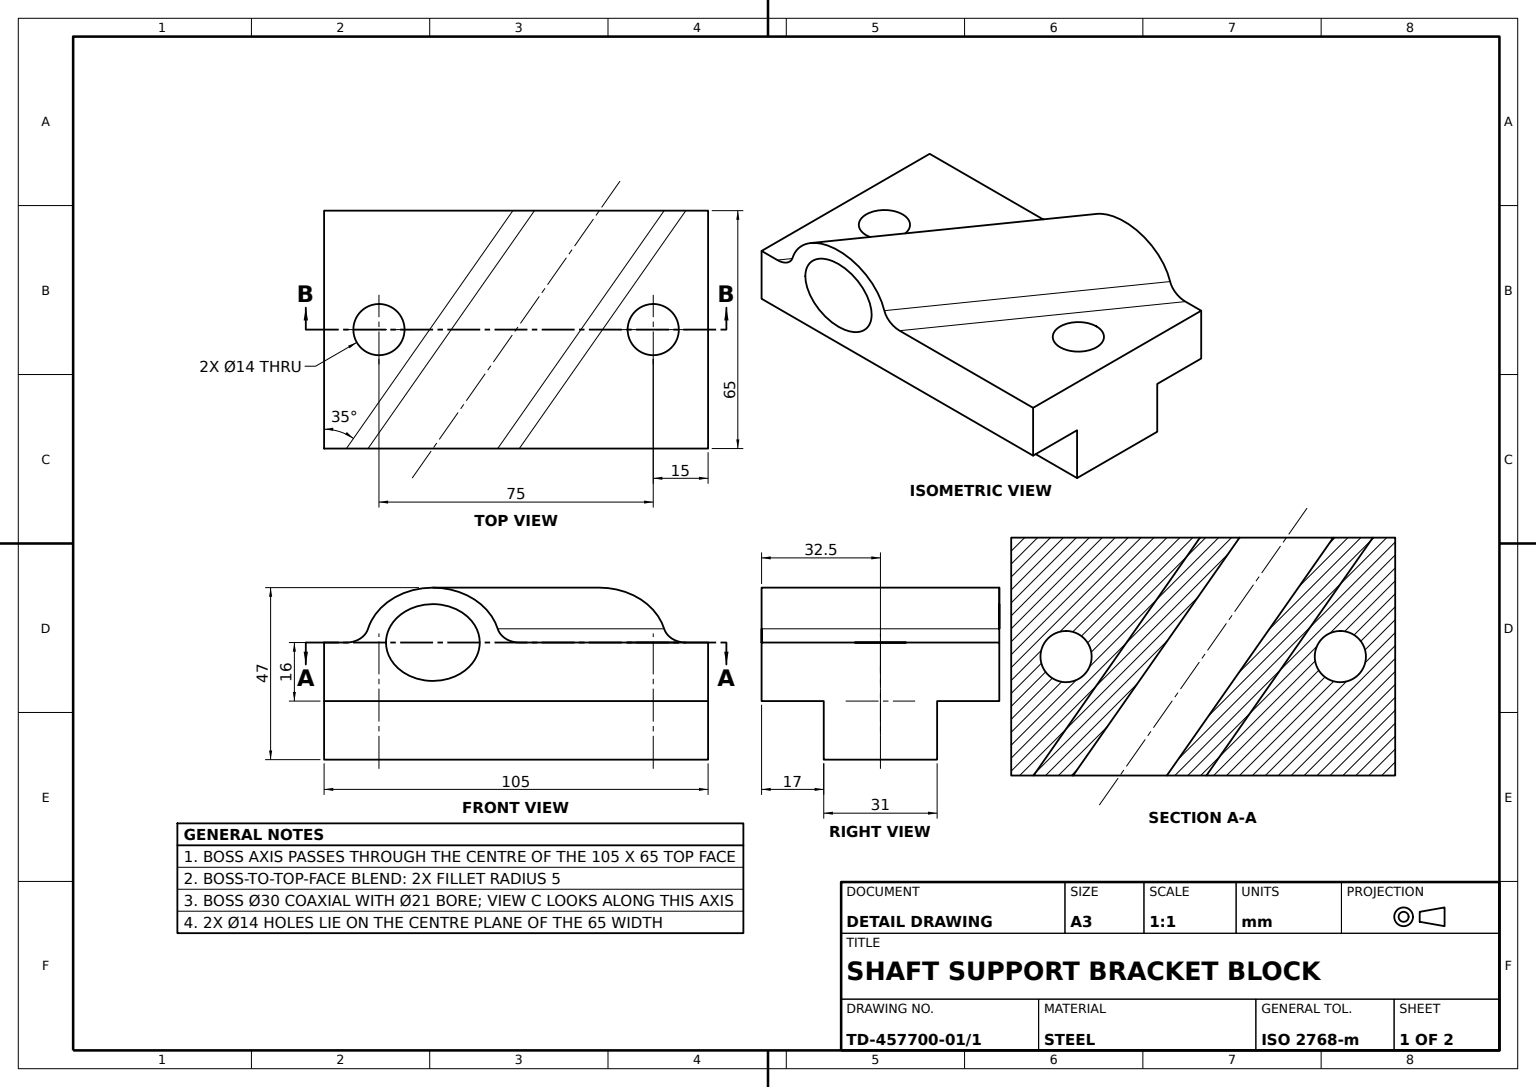
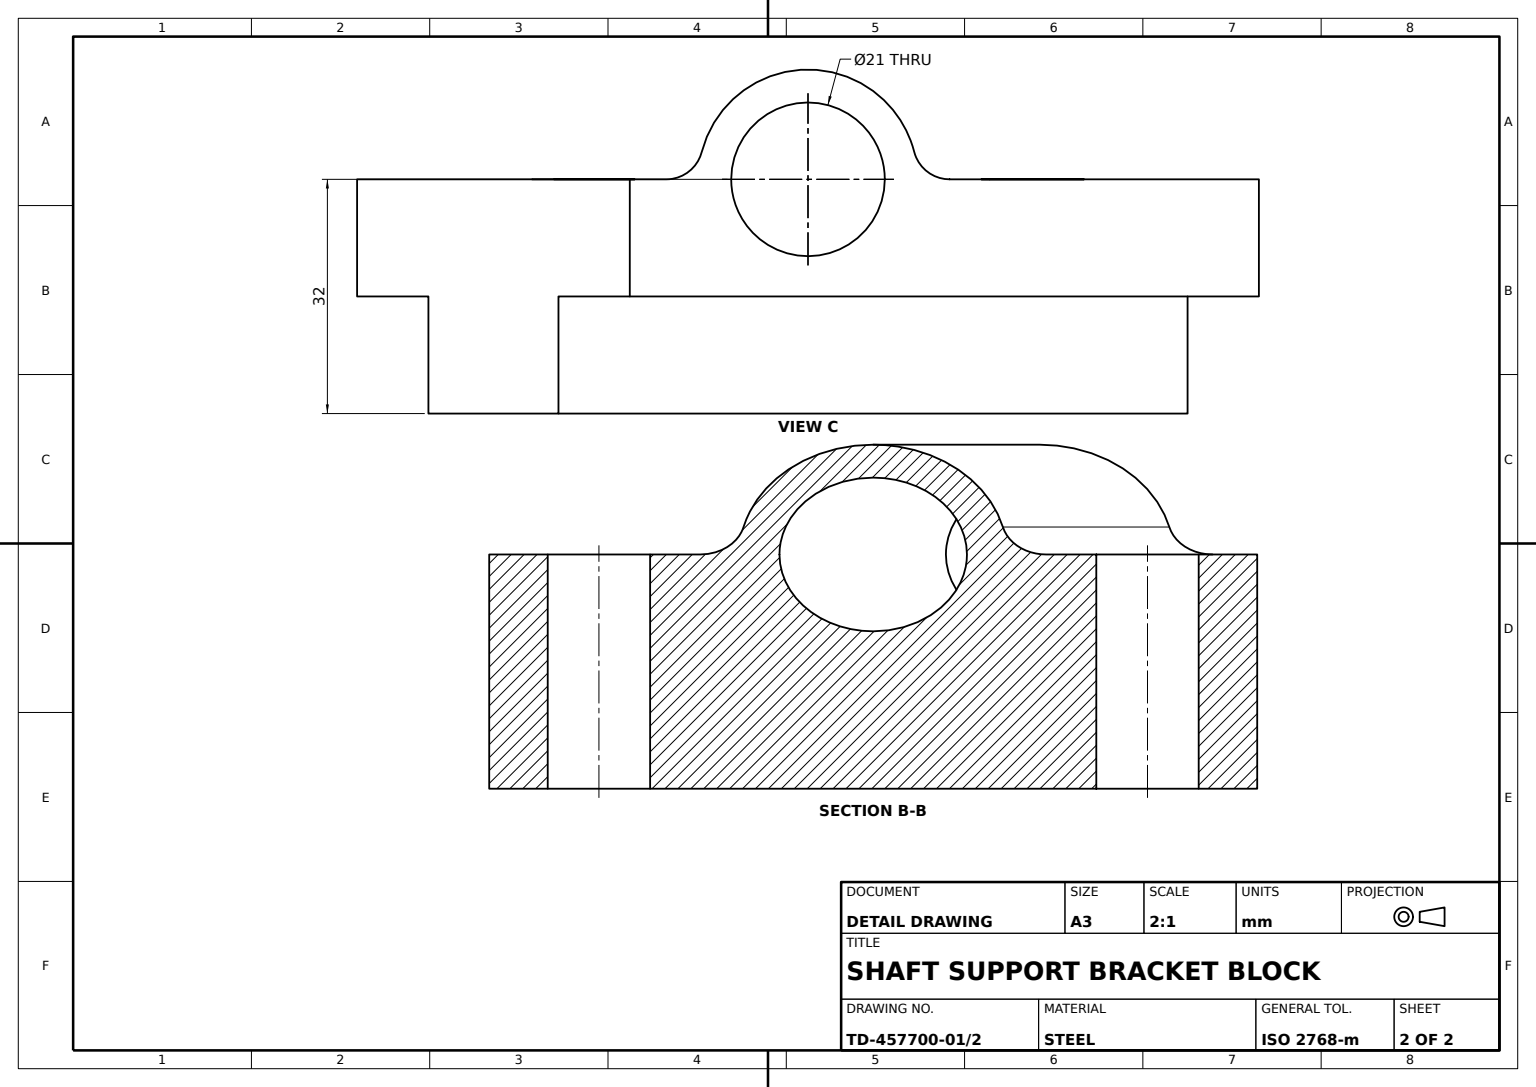
from build123d import *

# Parameters (mm, degrees)
BASE_PLATE_SKETCH_W                      = 105
BASE_PLATE_SKETCH_H                      = 65
BASE_PLATE_DEPTH                         = 16
LOCATING_KEY_SKETCH_W                    = 31
LOCATING_KEY_SKETCH_H                    = 16
LOCATING_KEY_DEPTH                       = 105
MOUNTING_HOLES_DEPTH                     = 70.544949493
MOUNTING_HOLES_DEPTH_BACK                = 70.544949493
MOUNTING_HOLES_SKETCH_R                  = 7
INCLINED_CYLINDER_BOSS_REACH             = 71.545
BOSS_PROFILE_SKETCH_R                    = 15
BOSS_PROFILE_SKETCH_R_2                  = 10.5
INCLINED_CYLINDER_BOSS_DIRECTION_2_REACH = 71.545
BOSS_BORE_DEPTH                          = 70.544949493
BOSS_BORE_DEPTH_BACK                     = 70.544949493
BOSS_BORE_SKETCH_R                       = 10.5
BOSS_BLEND_FILLET_R5_R                   = 5


with BuildPart() as part:
    # Base Plate Sketch → Base Plate (new body)
    with BuildSketch(Plane(origin=(0, 0, 0), x_dir=(1, 0, 0), z_dir=(0, 1, 0))):
        Rectangle(BASE_PLATE_SKETCH_W, BASE_PLATE_SKETCH_H)
    extrude(amount=-BASE_PLATE_DEPTH)

    # Locating Key Sketch → Locating Key (add)
    with BuildSketch(Plane.ZY.offset(52.5)):
        with Locations((0, -24)):
            Rectangle(LOCATING_KEY_SKETCH_W, LOCATING_KEY_SKETCH_H)
    extrude(amount=-LOCATING_KEY_DEPTH)

    # Mounting Holes Sketch → Mounting Holes (cut, two sides: drawn at the far end of the back side and taken through both)
    with BuildSketch(Plane(origin=(0, 0, 0), x_dir=(1, 0, 0), z_dir=(0, 1, 0)).offset(-MOUNTING_HOLES_DEPTH_BACK)):
        with Locations(Location((-37.5, 0, 0), (0, 0, 270))):
            Circle(MOUNTING_HOLES_SKETCH_R)
        with Locations(Location((37.5, 0, 0), (0, 0, 270))):
            Circle(MOUNTING_HOLES_SKETCH_R)
    extrude(amount=MOUNTING_HOLES_DEPTH + MOUNTING_HOLES_DEPTH_BACK, mode=Mode.SUBTRACT)

    # Inclined Cylinder Boss: up to this plane
    inclined_cylinder_boss_end = Plane(origin=(-52.5, -16, 32.5), z_dir=(0, 0, 1))
    # Boss Profile Sketch → Inclined Cylinder Boss (add, up to the surface)
    with BuildSketch(Plane(origin=(0, 0, 0), x_dir=(0.819152044288991, 0, 0.5735764363510473), z_dir=(-0.5735764363510473, 0, 0.819152044288991)), mode=Mode.PRIVATE) as inclined_cylinder_boss_sk1:
        Circle(BOSS_PROFILE_SKETCH_R)
        Circle(BOSS_PROFILE_SKETCH_R_2, mode=Mode.SUBTRACT)
    inclined_cylinder_boss_tool1 = split(extrude(inclined_cylinder_boss_sk1.sketch, amount=INCLINED_CYLINDER_BOSS_REACH, mode=Mode.PRIVATE), bisect_by=inclined_cylinder_boss_end, keep=Keep.BOTH, mode=Mode.PRIVATE)
    add(inclined_cylinder_boss_tool1.solids().sort_by_distance((-11.939744, 0, -8.360299))[0])

    # Inclined Cylinder Boss direction 2: up to this plane
    inclined_cylinder_boss_direction_2_end = Plane(origin=(-52.5, -16, -32.5), z_dir=(0, 0, -1))
    # Boss Profile Sketch → Inclined Cylinder Boss direction 2 (add, up to the surface)
    with BuildSketch(Plane(origin=(0, 0, 0), x_dir=(0.819152044288991, 0, 0.5735764363510473), z_dir=(-0.5735764363510473, 0, 0.819152044288991)), mode=Mode.PRIVATE) as inclined_cylinder_boss_direction_2_sk1:
        Circle(BOSS_PROFILE_SKETCH_R)
        Circle(BOSS_PROFILE_SKETCH_R_2, mode=Mode.SUBTRACT)
    inclined_cylinder_boss_direction_2_tool1 = split(extrude(inclined_cylinder_boss_direction_2_sk1.sketch, amount=-INCLINED_CYLINDER_BOSS_DIRECTION_2_REACH, mode=Mode.PRIVATE), bisect_by=inclined_cylinder_boss_direction_2_end, keep=Keep.BOTH, mode=Mode.PRIVATE)
    add(inclined_cylinder_boss_direction_2_tool1.solids().sort_by_distance((-11.939744, 0, -8.360299))[0])

    # Boss Bore Sketch → Boss Bore (cut, two sides: drawn at the far end of the back side and taken through both)
    with BuildSketch(Plane(origin=(0, 0, 0), x_dir=(0.819152044288991, 0, 0.5735764363510473), z_dir=(-0.5735764363510473, 0, 0.819152044288991)).offset(-BOSS_BORE_DEPTH_BACK)):
        with Locations(Location((0, 0, 0), (0, 0, 180))):
            Circle(BOSS_BORE_SKETCH_R)
    extrude(amount=BOSS_BORE_DEPTH + BOSS_BORE_DEPTH_BACK, mode=Mode.SUBTRACT)

    # Boss Blend Fillet R5
    boss_blend_fillet_r5_edges = [part.edges().sort_by_distance(p)[0] for p in [
        (-18.311618831, 0, 0),
        (18.311618831, 0, 0),
    ]]
    fillet(boss_blend_fillet_r5_edges, radius=BOSS_BLEND_FILLET_R5_R)


solid = part.part
